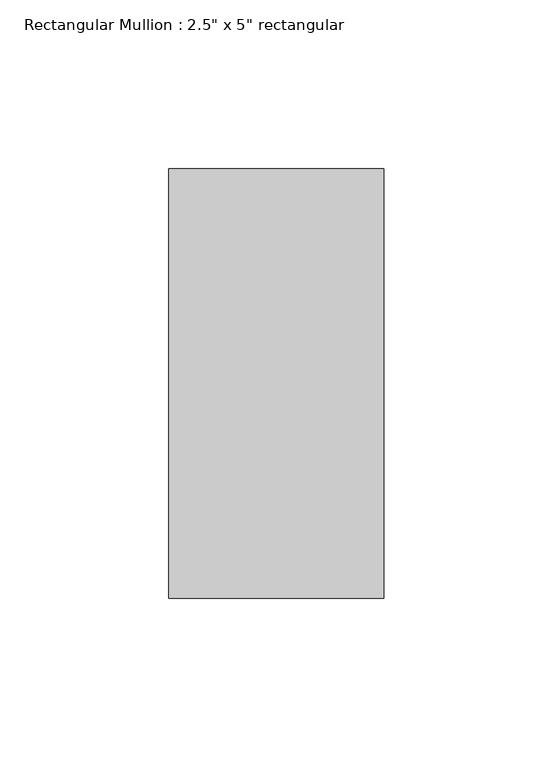
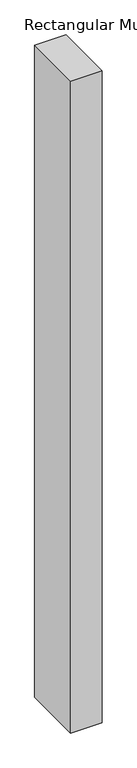
"""IFC4 building model written with IfcOpenShell, lengths in millimetres: member geometry."""

from ifc_helpers import new_model, si_unit, frame, origin, place, context, project, spatial, polyline, outline, extrude, source, transform, mapped, element, save


def member_09480567(model_context):
    return source(origin(), model_context, "Body", "SweptSolid", [
        extrude(outline(polyline([(0.0, 63.5), (0.0, -63.5), (-63.5, -63.5), (-63.5, 63.5), (0.0, 63.5)])), frame((0.0, 0.0, -1401.8499484), z_axis=(0.0, 0.0, 1.0), x_axis=(1.0, 0.0, 0.0)), (0.0, 0.0, 1.0), 1401.8499484),
    ])


if __name__ == "__main__":
    model = new_model("IFC4")
    model_context = context("Model", 3, world=origin())
    ifc_project = project(units=[si_unit("LENGTHUNIT", "METRE", prefix="MILLI")], contexts=[model_context])
    site = spatial("IfcSite", under=ifc_project)
    building = spatial("IfcBuilding", under=site)
    placement = place(None, origin())
    member_shape = member_09480567(model_context)
    element("IfcMember", 1, ObjectType="Rectangular Mullion : 2.5\" x 5\" rectangular", at=placement, inside=building, context=model_context, shape_type="MappedRepresentation", body=[
        mapped(member_shape, transform((0.0, 0.0, 0.0), x_axis=(1.0, 0.0, 0.0), y_axis=(0.0, 1.0, 0.0), z_axis=(0.0, 0.0, 1.0))),
    ])
    save(model, "model.ifc")

# Revit data of these elements
# Type "Rectangular Mullion : 2.5\" x 5\" rectangular"
#   built-in parameter 1007304 = 0.416667 (stored number, unit not read)
#   built-in parameter 1007301 = 0.104167 (stored number, unit not read)
#   built-in parameter 1007300 = 0.104167 (stored number, unit not read)
# Element 1 (IfcMember, "Rectangular Mullion : 2.5\" x 5\" rectangular")
#   Materials on its faces: "Aluminum"
# Materials
#   "Aluminum": class "Metal", colour RGB 247 247 247, transparency 0, Description = "Aluminum 6061", Cost = 0
